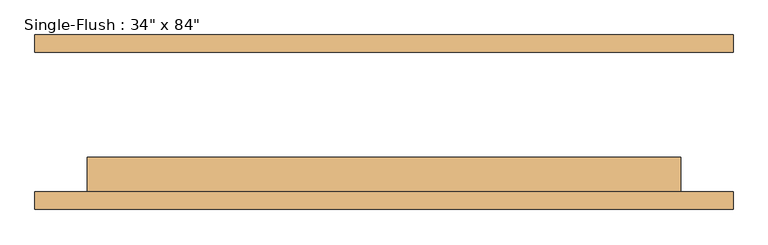
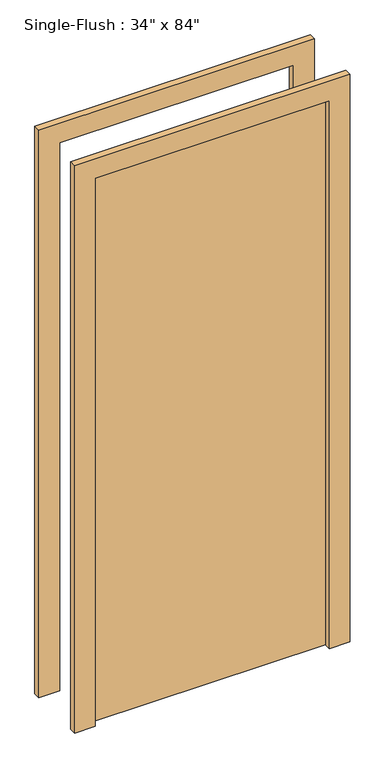
"""IFC4 building model written with IfcOpenShell, lengths in millimetres: door geometry."""

from ifc_helpers import new_model, si_unit, frame, origin, origin_with_axes, place, context, project, spatial, polyline, outline, extrude, source, transform, mapped, element, save


def door_74220ae7(model_context):
    return source(origin(), model_context, "Body", "SweptSolid", [
        extrude(outline(polyline([(2209.8, -508.0), (0.0, -508.0), (0.0, -431.8), (2133.6, -431.8), (2133.6, 431.8), (0.0, 431.8), (0.0, 508.0), (2209.8, 508.0), (2209.8, -508.0)])), frame((0.0, -127.0, 0.0), z_axis=(0.0, 1.0, 0.0), x_axis=(0.0, 0.0, 1.0)), (0.0, 0.0, 1.0), 25.4),
        extrude(outline(polyline([(2209.8, 508.0), (2209.8, -508.0), (0.0, -508.0), (0.0, -431.8), (2133.6, -431.8), (2133.6, 431.8), (0.0, 431.8), (0.0, 508.0), (2209.8, 508.0)])), frame((0.0, 101.6, 0.0), z_axis=(0.0, 1.0, 0.0), x_axis=(0.0, 0.0, 1.0)), (0.0, 0.0, 1.0), 25.4),
        extrude(outline(polyline([(431.8, -50.8), (431.8, -101.6), (-431.8, -101.6), (-431.8, -50.8), (431.8, -50.8)])), origin_with_axes(), (0.0, 0.0, 1.0), 2133.6),
    ])


if __name__ == "__main__":
    model = new_model("IFC4")
    model_context = context("Model", 3, world=origin())
    ifc_project = project(units=[si_unit("LENGTHUNIT", "METRE", prefix="MILLI")], contexts=[model_context])
    site = spatial("IfcSite", under=ifc_project)
    building = spatial("IfcBuilding", under=site)
    placement = place(None, origin())
    door_shape = door_74220ae7(model_context)
    element("IfcDoor", 1, ObjectType="Single-Flush : 34\" x 84\"", at=placement, inside=building, context=model_context, shape_type="MappedRepresentation", body=[
        mapped(door_shape, transform((0.0, 0.0, 0.0), x_axis=(1.0, 0.0, 0.0), y_axis=(0.0, 1.0, 0.0), z_axis=(0.0, 0.0, 1.0))),
    ])
    save(model, "model.ifc")

# Revit data of these elements
# Type "Single-Flush : 34\" x 84\""
#   Type Mark = "2"
#   Construction Type Id = "MDOOR"
#   Assembly Code = "C1020"
#   Analytic Construction = "Metal"
#   Thickness = 0' - 2"
#   Heat Transfer Coefficient (U) = 0.651978 BTU/(h·ft²·°F)
#   Height = 7' - 0"
#   Trim Projection Ext = 0' - 1"
#   Trim Projection Int = 0' - 1"
#   Trim Width = 0' - 3"
#   Width = 2' - 10"
#   Define Thermal Properties by = 1
#   Door Material = Door - Panel
#   Frame Material = Door - Frame
#   Visual Light Transmittance = 0
#   Solar Heat Gain Coefficient = 0
#   Function = (empty or 0)
#   Wall Closure = (empty or 0)
# Element 1 (IfcDoor, "Single-Flush : 34\" x 84\"")
#   Materials on its faces: "Door - Frame", "Door - Panel"
# Materials
#   "Door - Panel": class "Wood", colour RGB 210 159 95, transparency 0
#   "Door - Frame": colour RGB 118 70 51, transparency 0
